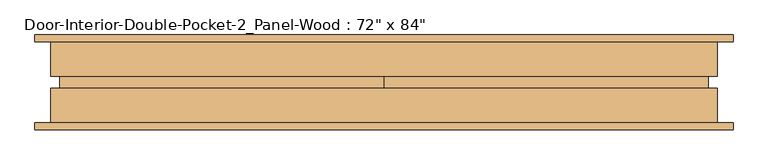
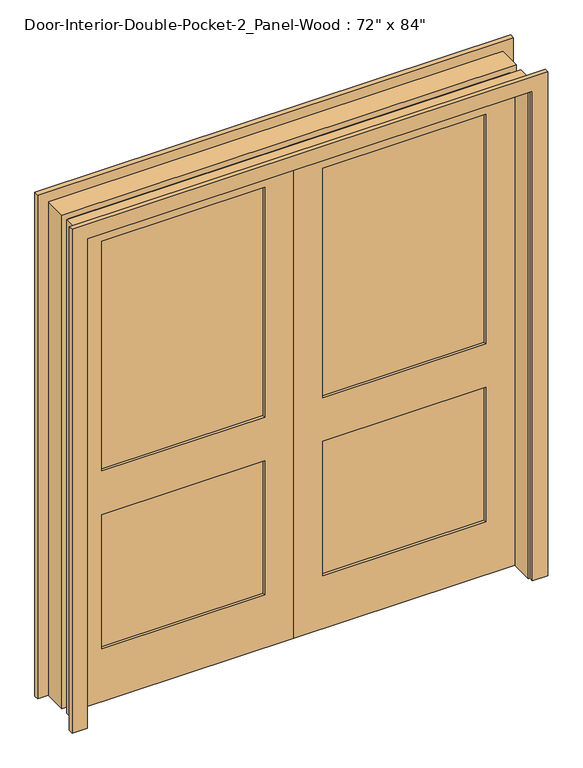
"""IFC4 building model written with IfcOpenShell, lengths in millimetres: door geometry."""

from ifc_helpers import new_model, si_unit, frame, origin, place, context, project, spatial, polyline, outline, extrude, source, transform, mapped, element, save


def door_c75fb906(model_context):
    return source(origin(), model_context, "Body", "SweptSolid", [
        extrude(outline(polyline([(0.0, 920.75), (0.0, 984.25), (2203.45, 984.25), (2203.45, -984.25), (0.0, -984.25), (0.0, -920.75), (2139.95, -920.75), (2139.95, 920.75), (0.0, 920.75)])), frame((0.0, 114.3, 0.0), z_axis=(0.0, 1.0, 0.0), x_axis=(0.0, 0.0, 1.0)), (0.0, 0.0, 1.0), 19.05),
        extrude(outline(polyline([(0.0, 920.75), (0.0, 984.25), (2203.45, 984.25), (2203.45, -984.25), (0.0, -984.25), (0.0, -920.75), (2139.95, -920.75), (2139.95, 920.75), (0.0, 920.75)])), frame((0.0, -133.35, 0.0), z_axis=(0.0, 1.0, 0.0), x_axis=(0.0, 0.0, 1.0)), (0.0, 0.0, 1.0), 19.05),
        extrude(outline(polyline([(2133.6, 0.0), (0.0, 0.0), (0.0, 914.4), (2133.6, 914.4), (2133.6, 0.0)]), holes=[polyline([(2014.5375, 120.65), (2014.5375, 793.75), (1009.65, 793.75), (1009.65, 120.65), (2014.5375, 120.65)]), polyline([(819.15, 120.65), (819.15, 793.75), (231.775, 793.75), (231.775, 120.65), (819.15, 120.65)])]), frame((0.0, -17.4625, 0.0), z_axis=(0.0, 1.0, 0.0), x_axis=(0.0, 0.0, 1.0)), (0.0, 0.0, 1.0), 34.925),
        extrude(outline(polyline([(793.75, -5.8208333), (120.65, -5.8208333), (120.65, 5.8208333), (793.75, 5.8208333), (793.75, -5.8208333)])), frame((0.0, 0.0, 1009.65), z_axis=(0.0, 0.0, 1.0), x_axis=(1.0, 0.0, 0.0)), (0.0, 0.0, 1.0), 1004.8875),
        extrude(outline(polyline([(793.75, -5.8208333), (120.65, -5.8208333), (120.65, 5.8208333), (793.75, 5.8208333), (793.75, -5.8208333)])), frame((0.0, 0.0, 231.775), z_axis=(0.0, 0.0, 1.0), x_axis=(1.0, 0.0, 0.0)), (0.0, 0.0, 1.0), 587.375),
        extrude(outline(polyline([(0.0, 939.8), (2159.0, 939.8), (2159.0, -939.8), (0.0, -939.8), (0.0, -914.4), (2133.6, -914.4), (2133.6, 914.4), (0.0, 914.4), (0.0, 939.8)])), frame((0.0, 17.4625, 0.0), z_axis=(0.0, 1.0, 0.0), x_axis=(0.0, 0.0, 1.0)), (0.0, 0.0, 1.0), 96.8375),
        extrude(outline(polyline([(0.0, 939.8), (2159.0, 939.8), (2159.0, -939.8), (0.0, -939.8), (0.0, -914.4), (2133.6, -914.4), (2133.6, 914.4), (0.0, 914.4), (0.0, 939.8)])), frame((0.0, -114.3, 0.0), z_axis=(0.0, 1.0, 0.0), x_axis=(0.0, 0.0, 1.0)), (0.0, 0.0, 1.0), 96.8375),
        extrude(outline(polyline([(2133.6, -914.4), (0.0, -914.4), (0.0, 0.0), (2133.6, 0.0), (2133.6, -914.4)]), holes=[polyline([(2014.5375, -793.75), (2014.5375, -120.65), (1009.65, -120.65), (1009.65, -793.75), (2014.5375, -793.75)]), polyline([(819.15, -793.75), (819.15, -120.65), (231.775, -120.65), (231.775, -793.75), (819.15, -793.75)])]), frame((0.0, -17.4625, 0.0), z_axis=(0.0, 1.0, 0.0), x_axis=(0.0, 0.0, 1.0)), (0.0, 0.0, 1.0), 34.925),
        extrude(outline(polyline([(-120.65, -5.8208333), (-793.75, -5.8208333), (-793.75, 5.8208333), (-120.65, 5.8208333), (-120.65, -5.8208333)])), frame((0.0, 0.0, 1009.65), z_axis=(0.0, 0.0, 1.0), x_axis=(1.0, 0.0, 0.0)), (0.0, 0.0, 1.0), 1004.8875),
        extrude(outline(polyline([(-120.65, -5.8208333), (-793.75, -5.8208333), (-793.75, 5.8208333), (-120.65, 5.8208333), (-120.65, -5.8208333)])), frame((0.0, 0.0, 231.775), z_axis=(0.0, 0.0, 1.0), x_axis=(1.0, 0.0, 0.0)), (0.0, 0.0, 1.0), 587.375),
    ])


if __name__ == "__main__":
    model = new_model("IFC4")
    model_context = context("Model", 3, world=origin())
    ifc_project = project(units=[si_unit("LENGTHUNIT", "METRE", prefix="MILLI")], contexts=[model_context])
    site = spatial("IfcSite", under=ifc_project)
    building = spatial("IfcBuilding", under=site)
    placement = place(None, origin())
    door_shape = door_c75fb906(model_context)
    element("IfcDoor", 1, ObjectType="Door-Interior-Double-Pocket-2_Panel-Wood : 72\" x 84\"", at=placement, inside=building, context=model_context, shape_type="MappedRepresentation", body=[
        mapped(door_shape, transform((0.0, 0.0, 0.0), x_axis=(1.0, 0.0, 0.0), y_axis=(0.0, 1.0, 0.0), z_axis=(0.0, 0.0, 1.0))),
    ])
    save(model, "model.ifc")

# Revit data of these elements
# Type "Door-Interior-Double-Pocket-2_Panel-Wood : 72\" x 84\""
#   Type Mark = "8"
#   Assembly Code = "C1020300"
#   Analytic Construction = "Wooden"
#   Top Rail = 0' - 4 11/16"
#   Thickness = 0' - 1 3/8"
#   Thermal Resistance (R) = 2.5876 (h·ft²·°F)/BTU
#   Stiles = 0' - 4 3/4"
#   Rough Width = 12' - 2"
#   Rough Height = 7' - 4 1/2"
#   Panel Width = 3' - 0"
#   Lock Rail = 0' - 7 1/2"
#   Location [instance default] = 3' - 1"
#   Height = 7' - 0"
#   Width = 6' - 0"
#   Heat Transfer Coefficient (U) = 0.3865 BTU/(h·ft²·°F)
#   Bottom Rail = 0' - 9 1/8"
#   Panel Open [instance default] = no
#   Trim Material = Cherry
#   Panel Material = door wood colour
#   Frame Material = door wood colour
#   Visual Light Transmittance = 0
#   Solar Heat Gain Coefficient = 0
#   Wall Closure = (empty or 0)
#   Function = (empty or 0)
# Element 1 (IfcDoor, "Door-Interior-Double-Pocket-2_Panel-Wood : 72\" x 84\"")
#   Materials on its faces: "door wood colour", "Cherry"
# Materials
#   "Cherry": class "Wood", colour RGB 226 177 128, transparency 0, Description = "Prunus Serotina", Cost = 0
#   "door wood colour": class "Generic", colour RGB 120 120 120, transparency 0, Cost = 0
